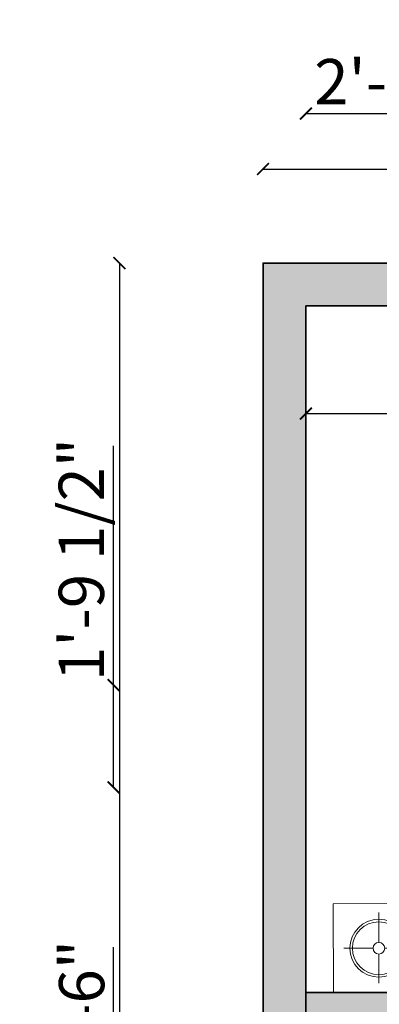
# Model space of a CAD drawing. Units: inches. Extents: x 1704 to 2334, y 1856 to 2559.
# Tile 4 of 10: x 1704 to 1779, y 2353 to 2559. Entities that reach past the tile are written whole.
import ezdxf

# ---------------------------------------------------------------- set-up
doc = ezdxf.new("R2010")
doc.units = ezdxf.units.IN
for name, color, linetype, lineweight in [('A-ANNO-DIMS', 2, 'Continuous', 18), ('A-WALL', 7, 'Continuous', 35), ('BEDS', 17, 'Continuous', 18)]:
    doc.layers.add(name, color=color, linetype=linetype, lineweight=lineweight)
doc.layers.add('A-WALL-PATT', color=18, linetype='Continuous', lineweight=13, true_color=0x000000)
doc.styles.get("Standard").update_dxf_attribs({"font": 'arial.ttf'})
doc.dimstyles.new('ISO-25', dxfattribs={"dimtxt": 9.5, "dimasz": 2.5, "dimexe": 1.25, "dimexo": 0.625, "dimtad": 1, "dimdec": 0, "dimlunit": 4, "dimtxsty": 'Standard', "dimblk": 'ARCHTICK', "dimcen": 2.5, "dimse1": 1, "dimse2": 1, "dimclrd": 3, "dimadec": 0, "dimazin": 0, "dimtfac": 1, "dimtdec": 0, "dimtmove": 0, "dimatfit": 3, "dimfxl": 1, "dimarcsym": 0})

# ---------------------------------------------------------------- blocks, each defined once
blk = doc.blocks.new('A$C77DF40FE')
for p, q in [((0.5, 2.6723), (0, 2.6723)), ((0, 2.6723), (0, 2.1723)), ((0.226, 2.4949), (0.226, 2.6594)), ((0.5, 2.1723), (0.5, 2.6723)), ((0.5839, 2.6714), (2.0097, 2.6714)), ((2.0936, 2.1723), (2.0936, 2.6723)), ((2.0936, 2.6723), (2.5936, 2.6723)), ((2.5936, 2.6723), (2.5936, 2.1723)), ((0.5339, 0.6344), (0.5339, 2.6214)), ((0.5839, 2.6214), (2.0097, 2.6214)), ((0.5839, 0.6344), (0.5839, 2.6214)), ((2.0097, 2.6214), (2.0097, 0.6344)), ((2.0597, 2.6214), (2.0597, 0.6344)), ((2.3379, 2.4554), (2.3379, 2.6199)), ((0.6508, 2.5603), (0.6508, 2.2403)), ((1.2408, 2.5803), (0.6708, 2.5803)), ((1.2608, 2.2403), (1.2608, 2.5603)), ((1.3355, 2.5603), (1.3355, 2.2403)), ((1.9255, 2.5803), (1.3555, 2.5803)), ((1.9455, 2.2403), (1.9455, 2.5603)), ((0.0287, 2.4621), (0.1932, 2.4621)), ((0.2588, 2.4621), (0.4233, 2.4621)), ((0.226, 2.261), (0.226, 2.4293)), ((0.4809, 2.3823), (0.4746, 2.3757)), ((0.4873, 2.387), (0.4809, 2.3823)), ((0.4937, 2.3899), (0.4873, 2.387)), ((0.5, 2.3914), (0.4937, 2.3899)), ((0.506, 2.3917), (0.5, 2.3914)), ((0.5117, 2.391), (0.506, 2.3917)), ((0.5168, 2.3897), (0.5117, 2.391)), ((0.5212, 2.3878), (0.5168, 2.3897)), ((0.5205, 2.3816), (0.5202, 2.3804)), ((0.5202, 2.3804), (0.5202, 2.379)), ((0.5202, 2.379), (0.5206, 2.3777)), ((0.521, 2.3828), (0.5205, 2.3816)), ((0.5219, 2.3839), (0.521, 2.3828)), ((0.5248, 2.3858), (0.5212, 2.3878)), ((0.523, 2.3849), (0.5219, 2.3839)), ((0.5244, 2.3856), (0.523, 2.3849)), ((0.5261, 2.3861), (0.5244, 2.3856)), ((0.5277, 2.3836), (0.5248, 2.3858)), ((0.5279, 2.3864), (0.5261, 2.3861)), ((0.5298, 2.3813), (0.5277, 2.3836)), ((0.5298, 2.3864), (0.5279, 2.3864)), ((0.5318, 2.3861), (0.5298, 2.3864)), ((0.5313, 2.3792), (0.5298, 2.3813)), ((0.5322, 2.3771), (0.5313, 2.3792)), ((0.5338, 2.3855), (0.5318, 2.3861)), ((0.5356, 2.3846), (0.5338, 2.3855)), ((0.5373, 2.3832), (0.5356, 2.3846)), ((0.5387, 2.3815), (0.5373, 2.3832)), ((0.5399, 2.3794), (0.5387, 2.3815)), ((0.5407, 2.377), (0.5399, 2.3794)), ((2.3051, 2.4226), (2.1406, 2.4226)), ((2.3379, 2.2215), (2.3379, 2.3898)), ((2.5352, 2.4226), (2.3707, 2.4226)), ((0.2338, 2.3688, 10.4), (0.2338, 2.1957, 10.4)), ((0.4828, 2.3788, 10.4), (0.2438, 2.3788, 10.4)), ((0.2538, 2.353, 10.4), (0.2538, 2.3215, 10.4)), ((0.4656, 2.363, 10.4), (0.2638, 2.363, 10.4)), ((0.4756, 2.3215, 10.4), (0.4756, 2.353, 10.4)), ((0.4767, 2.3409), (0.4876, 2.34)), ((0.4876, 2.34), (0.4961, 2.3402)), ((0.4928, 2.1957, 10.4), (0.4928, 2.3688, 10.4)), ((0.4961, 2.3402), (0.5023, 2.3413)), ((0.502, 2.3463), (0.5017, 2.3431)), ((0.5017, 2.3431), (0.5018, 2.3398)), ((0.5018, 2.3398), (0.5023, 2.3365)), ((0.5026, 2.3491), (0.502, 2.3463)), ((0.5023, 2.3413), (0.5067, 2.3431)), ((0.5023, 2.3365), (0.5031, 2.3334)), ((0.5035, 2.3514), (0.5026, 2.3491)), ((0.5031, 2.3334), (0.5043, 2.3309)), ((0.5047, 2.3531), (0.5035, 2.3514)), ((0.5043, 2.3309), (0.506, 2.329)), ((0.5059, 2.3542), (0.5047, 2.3531)), ((0.5073, 2.3548), (0.5059, 2.3542)), ((0.506, 2.329), (0.5081, 2.328)), ((0.5067, 2.3431), (0.5095, 2.3452)), ((0.5086, 2.3549), (0.5073, 2.3548)), ((0.5081, 2.328), (0.5106, 2.328)), ((0.5097, 2.3544), (0.5086, 2.3549)), ((0.5095, 2.3452), (0.511, 2.3475)), ((0.5107, 2.3534), (0.5097, 2.3544)), ((0.5106, 2.328), (0.5134, 2.3288)), ((0.5113, 2.3518), (0.5107, 2.3534)), ((0.511, 2.3475), (0.5115, 2.3498)), ((0.5115, 2.3498), (0.5113, 2.3518)), ((0.5134, 2.3288), (0.5163, 2.3304)), ((0.5163, 2.3304), (0.5193, 2.3325)), ((0.5193, 2.3325), (0.5222, 2.3349)), ((0.5206, 2.3777), (0.5213, 2.3764)), ((0.5213, 2.3764), (0.5224, 2.3752)), ((0.5222, 2.3349), (0.5249, 2.3374)), ((0.5224, 2.3752), (0.5237, 2.374)), ((0.5237, 2.374), (0.5252, 2.3731)), ((0.5249, 2.3374), (0.5271, 2.3398)), ((0.5252, 2.3731), (0.5268, 2.3723)), ((0.5268, 2.3723), (0.5283, 2.3719)), ((0.5271, 2.3398), (0.5288, 2.3419)), ((0.5283, 2.3719), (0.5297, 2.3717)), ((0.5288, 2.3419), (0.5299, 2.3436)), ((0.5297, 2.3717), (0.531, 2.372)), ((0.5299, 2.3436), (0.5305, 2.3449)), ((0.53, 2.3482), (0.5302, 2.3488)), ((0.5301, 2.3477), (0.53, 2.3482)), ((0.5303, 2.3472), (0.5301, 2.3477)), ((0.5302, 2.3488), (0.5308, 2.3495)), ((0.5306, 2.3466), (0.5303, 2.3472)), ((0.5305, 2.3449), (0.5307, 2.3459)), ((0.5307, 2.3459), (0.5306, 2.3466)), ((0.5308, 2.3495), (0.5317, 2.3504)), ((0.531, 2.372), (0.5319, 2.3726)), ((0.5317, 2.3504), (0.5329, 2.3515)), ((0.5319, 2.3726), (0.5325, 2.3738)), ((0.5326, 2.3753), (0.5322, 2.3771)), ((0.5325, 2.3738), (0.5326, 2.3753)), ((0.5329, 2.3515), (0.5342, 2.3528)), ((0.5342, 2.3528), (0.5356, 2.3543)), ((0.5356, 2.3543), (0.537, 2.3561)), ((0.537, 2.3561), (0.5383, 2.3581)), ((0.5383, 2.3581), (0.5394, 2.3604)), ((0.5394, 2.3604), (0.5403, 2.3629)), ((0.5403, 2.3629), (0.5409, 2.3657)), ((0.5412, 2.3743), (0.5407, 2.377)), ((0.5409, 2.3657), (0.5413, 2.3686)), ((0.5414, 2.3715), (0.5412, 2.3743)), ((0.5413, 2.3686), (0.5414, 2.3715)), ((0.2638, 2.3115, 10.4), (0.4656, 2.3115, 10.4)), ((0.6708, 2.2203), (1.2408, 2.2203)), ((1.3555, 2.2203), (1.9255, 2.2203)), ((0, 2.1723), (0.5, 2.1723)), ((0.2438, 2.1857, 10.4), (0.4828, 2.1857, 10.4)), ((2.5936, 2.1723), (2.0936, 2.1723)), ((1.5773, 2.1205), (1.0147, 2.1205)), ((0.1072, 1.9057), (0.0269, 1.9485)), ((0.0644, 1.9807), (0.1019, 1.9003)), ((0.1072, 1.986), (0.1072, 1.911)), ((0.134, 1.9753), (0.134, 1.9057)), ((0.1554, 1.9914), (0.1554, 1.911)), ((0.1792, 1.9138), (0.1849, 1.9847)), ((0.2134, 1.9138), (0.219, 1.9847)), ((0.251, 1.9118), (0.2494, 1.9865)), ((0.2748, 1.9118), (0.2691, 1.9849)), ((0.2899, 1.9138), (0.2956, 1.9847)), ((0.3277, 1.9118), (0.3219, 1.9849)), ((0.3539, 1.9118), (0.3522, 1.9865)), ((0.3766, 1.9138), (0.3822, 1.9847)), ((0.4142, 1.9118), (0.4126, 1.9865)), ((0.438, 1.9118), (0.4323, 1.9849)), ((0.4531, 1.9138), (0.4588, 1.9847)), ((0.4873, 1.9138), (0.493, 1.9847)), ((0.5249, 1.9118), (0.5233, 1.9865)), ((0.0195, 1.8887), (0.0942, 1.8903)), ((0.1019, 1.9003), (0.0269, 1.9003)), ((0.1002, 1.8885), (0.1002, 0.0935)), ((0.3112, 1.9057), (0.1019, 1.9057)), ((0.1019, 1.9057), (0.1019, 1.8628)), ((0.5301, 1.9057), (0.3112, 1.9057)), ((0.6051, 1.925), (0.7457, 1.7234)), ((1.9869, 1.925), (1.8463, 1.7234)), ((0.0227, 1.8712), (0.0957, 1.8769)), ((0.0247, 1.8561), (0.0955, 1.8504)), ((0.0227, 1.7843), (0.0974, 1.786)), ((0.0247, 1.8219), (0.0955, 1.8163)), ((0.3112, 1.8116), (0.1852, 1.8116)), ((0.1852, 1.8116), (0.1852, 0.187)), ((0.3112, 1.7816), (0.2152, 1.7816)), ((0.2152, 1.7816), (0.2152, 0.217)), ((0.5339, 1.8116), (0.3112, 1.8116)), ((0.5339, 1.7816), (0.3112, 1.7816)), ((0.3909, 1.7821), (0.5339, 1.398)), ((0.0227, 1.7605), (0.0957, 1.7662)), ((0.0247, 1.7454), (0.0955, 1.7397)), ((0.0247, 1.708), (0.0955, 1.7023)), ((0.0247, 1.6819), (0.0955, 1.6762)), ((0.0227, 1.6443), (0.0974, 1.6459)), ((0.0227, 1.6205), (0.0957, 1.6262)), ((0.0247, 1.6054), (0.0955, 1.5997)), ((0.0227, 1.5505), (0.0974, 1.5521)), ((0.0247, 1.5881), (0.0955, 1.5824)), ((0.0227, 1.5266), (0.0957, 1.5324)), ((0.0247, 1.5116), (0.0955, 1.5059)), ((0.0227, 1.4397), (0.0974, 1.4414)), ((0.0247, 1.4774), (0.0955, 1.4717)), ((0.0227, 1.4159), (0.0957, 1.4217)), ((0.0247, 1.4008), (0.0955, 1.3952)), ((0.0247, 1.3634), (0.0955, 1.3577)), ((0.0247, 1.3374), (0.0955, 1.3317)), ((0.0227, 1.2997), (0.0974, 1.3014)), ((0.0227, 1.2759), (0.0957, 1.2816)), ((0.0247, 1.2608), (0.0955, 1.2551)), ((0.0247, 1.2266), (0.0955, 1.221)), ((0.0227, 1.189), (0.0974, 1.1906)), ((0.0227, 1.1652), (0.0957, 1.1709)), ((0.0227, 1.1414), (0.0957, 1.1471)), ((0.0247, 1.1163), (0.0955, 1.1106)), ((0.5339, 1.1132), (0.2152, 1.1479)), ((0.0227, 1.0786), (0.0974, 1.0803)), ((0.0227, 1.0548), (0.0957, 1.0606)), ((0.0247, 1.0397), (0.0955, 1.0341)), ((0.0247, 1.0055), (0.0955, 0.9999)), ((0.5339, 0.7837), (0.2152, 1.0221)), ((0.0227, 0.9679), (0.0974, 0.9696)), ((0.0227, 0.9441), (0.0957, 0.9498)), ((0.0247, 0.929), (0.0955, 0.9233)), ((0.0247, 0.8916), (0.0955, 0.8859)), ((0.0247, 0.8655), (0.0955, 0.8599)), ((0.0227, 0.8279), (0.0974, 0.8295)), ((0.0227, 0.8041), (0.0957, 0.8098)), ((0.0247, 0.789), (0.0955, 0.7833)), ((0.0247, 0.7548), (0.0955, 0.7491)), ((0.0227, 0.7172), (0.0974, 0.7188)), ((0.0227, 0.6933), (0.0957, 0.6991)), ((0.0247, 0.6783), (0.0955, 0.6726)), ((0.0247, 0.6408), (0.0955, 0.6352)), ((2.0097, 0.6344), (0.5839, 0.6344)), ((0.0227, 0.6032), (0.0974, 0.6048)), ((0.0227, 0.5794), (0.0957, 0.5851)), ((0.0247, 0.5643), (0.0955, 0.5586)), ((2.0097, 0.5844), (0.5839, 0.5844)), ((1.2963, 0.2134), (0.8003, 0.5844)), ((0.8369, 0.5844), (0.975, 0.2134)), ((1.6139, 0.217), (1.6139, 0.5844)), ((1.6439, 0.187), (1.6439, 0.5844)), ((1.7439, 0.087), (1.7439, 0.5844)), ((1.8197, 0.5605), (1.7489, 0.5548)), ((0.0247, 0.5301), (0.0955, 0.5244)), ((1.8218, 0.5229), (1.7471, 0.5245)), ((1.8218, 0.499), (1.7487, 0.5048)), ((0.0227, 0.4925), (0.0974, 0.4941)), ((0.0227, 0.4687), (0.0957, 0.4744)), ((0.0247, 0.4536), (0.0955, 0.4479)), ((1.8197, 0.4839), (1.7489, 0.4783)), ((1.8197, 0.453), (1.7489, 0.4474)), ((0.0247, 0.4227), (0.0955, 0.417)), ((1.8197, 0.4168), (1.7489, 0.4111)), ((0.0227, 0.3367), (0.0957, 0.3424)), ((0.0247, 0.3864), (0.0955, 0.3807)), ((1.8218, 0.3671), (1.7487, 0.3728)), ((1.8197, 0.352), (1.7489, 0.3463)), ((0.0247, 0.3216), (0.0955, 0.3159)), ((0.0247, 0.2842), (0.0955, 0.2785)), ((1.8197, 0.3146), (1.7489, 0.3089)), ((1.7492, 0.2844), (1.8223, 0.2787)), ((0.0227, 0.2465), (0.0974, 0.2482)), ((0.0227, 0.2227), (0.0957, 0.2285)), ((1.7492, 0.2606), (1.824, 0.2589)), ((1.7513, 0.223), (1.8221, 0.2286)), ((0.1019, 0.1857), (0.0216, 0.1857)), ((0.0247, 0.2076), (0.0955, 0.202)), ((0.1852, 0.187), (0.3112, 0.187)), ((0.2152, 0.217), (0.3112, 0.217)), ((0.3112, 0.217), (1.6139, 0.217)), ((0.3112, 0.187), (1.6439, 0.187)), ((1.7492, 0.1737), (1.8223, 0.1679)), ((1.7513, 0.1888), (1.8221, 0.1944)), ((0.1019, 0.1535), (0.0269, 0.1482)), ((0.1019, 0.116), (0.0269, 0.1214)), ((1.7492, 0.1499), (1.824, 0.1482)), ((1.7513, 0.1122), (1.8221, 0.1179)), ((0.0965, 0.0946), (0.0269, 0.0303)), ((0.1019, 0.0892), (0.0269, 0.0892)), ((0.1019, 0.0946), (0.0751, 0.0089)), ((0.1002, 0.0935), (0.3112, 0.0935)), ((0.107, 0.0096), (0.1126, 0.0804)), ((0.1446, 0.0075), (0.1429, 0.0823)), ((0.1684, 0.0075), (0.1627, 0.0806)), ((0.1835, 0.0096), (0.1892, 0.0804)), ((0.2209, 0.0096), (0.2266, 0.0804)), ((0.247, 0.0096), (0.2527, 0.0804)), ((0.2846, 0.0075), (0.283, 0.0823)), ((0.3084, 0.0075), (0.3027, 0.0806)), ((0.3112, 0.0935), (1.0155, 0.0935)), ((0.3151, 0.0075), (0.3112, 0.0565)), ((0.3301, 0.0096), (0.3358, 0.0804)), ((0.3676, 0.0096), (0.3732, 0.0804)), ((0.3936, 0.0096), (0.3993, 0.0804)), ((0.4313, 0.0075), (0.4296, 0.0823)), ((0.4551, 0.0075), (0.4493, 0.0806)), ((0.4702, 0.0096), (0.4758, 0.0804)), ((0.5043, 0.0096), (0.51, 0.0804)), ((0.542, 0.0075), (0.5403, 0.0823)), ((0.5658, 0.0075), (0.56, 0.0806)), ((0.5896, 0.0075), (0.5838, 0.0806)), ((0.6147, 0.0096), (0.6204, 0.0804)), ((0.6523, 0.0075), (0.6507, 0.0823)), ((0.6762, 0.0075), (0.6704, 0.0806)), ((0.6912, 0.0096), (0.6969, 0.0804)), ((0.7254, 0.0096), (0.7311, 0.0804)), ((0.7631, 0.0075), (0.7614, 0.0823)), ((0.7869, 0.0075), (0.7811, 0.0806)), ((0.802, 0.0096), (0.8076, 0.0804)), ((0.8394, 0.0096), (0.8451, 0.0804)), ((0.8654, 0.0096), (0.8711, 0.0804)), ((0.9031, 0.0075), (0.9014, 0.0823)), ((0.9269, 0.0075), (0.9212, 0.0806)), ((0.942, 0.0096), (0.9477, 0.0804)), ((0.9762, 0.0096), (0.9818, 0.0804)), ((1.0138, 0.0075), (1.0122, 0.0823)), ((1.0155, 0.0935), (1.7355, 0.0935)), ((1.0376, 0.0075), (1.0319, 0.0806)), ((1.0527, 0.0096), (1.0584, 0.0804)), ((1.0901, 0.0096), (1.0958, 0.0804)), ((1.1278, 0.0075), (1.1261, 0.0823)), ((1.1516, 0.0075), (1.1459, 0.0806)), ((1.1667, 0.0096), (1.1724, 0.0804)), ((1.2009, 0.0096), (1.2065, 0.0804)), ((1.2385, 0.0075), (1.2368, 0.0823)), ((1.2623, 0.0075), (1.2566, 0.0806)), ((1.2774, 0.0096), (1.2831, 0.0804)), ((1.3083, 0.0096), (1.314, 0.0804)), ((1.3446, 0.0096), (1.3503, 0.0804)), ((1.3943, 0.0075), (1.3885, 0.0806)), ((1.4094, 0.0096), (1.415, 0.0804)), ((1.4468, 0.0096), (1.4525, 0.0804)), ((1.4844, 0.0075), (1.4828, 0.0823)), ((1.5083, 0.0075), (1.5025, 0.0806)), ((1.5233, 0.0096), (1.529, 0.0804)), ((1.5575, 0.0096), (1.5632, 0.0804)), ((1.5951, 0.0075), (1.5935, 0.0823)), ((1.619, 0.0075), (1.6132, 0.0806)), ((1.6341, 0.0096), (1.6397, 0.0804)), ((1.665, 0.0096), (1.6706, 0.0804)), ((1.6831, 0.0096), (1.6888, 0.0804)), ((1.7162, 0.0857), (1.7162, 0)), ((1.7323, 0.0911), (1.7269, 0.0107)), ((1.743, 0.0857), (1.8126, 0.0054)), ((1.7483, 0.0911), (1.8233, 0.0322)), ((1.7483, 0.0857), (1.7537, 0.0054)), ((1.7513, 0.0858), (1.8221, 0.0915))]:
    blk.add_line(p, q)
for centre, radius in [((0.226, 2.4621), 0.1629), ((0.226, 2.4621), 0.1484), ((2.3379, 2.4226), 0.1629), ((2.3379, 2.4226), 0.1484), ((0.226, 2.4621), 0.0328), ((2.3379, 2.4226), 0.0328), ((0.2896, 2.2801, 10.4), 0.00858), ((0.3196, 2.2801, 10.4), 0.00858), ((0.3554, 2.2801, 10.4), 0.00858), ((0.3855, 2.2801, 10.4), 0.00858), ((0.2896, 2.25, 10.4), 0.00858), ((0.2896, 2.2186, 10.4), 0.00858), ((0.3196, 2.25, 10.4), 0.00858), ((0.3196, 2.2186, 10.4), 0.00858), ((0.3554, 2.25, 10.4), 0.00858), ((0.3554, 2.2186, 10.4), 0.00858), ((0.3855, 2.25, 10.4), 0.00858), ((0.3855, 2.2186, 10.4), 0.00858)]:
    blk.add_circle(centre, radius)
for centre, radius, start, end in [((0.5839, 2.6214), 0.05, 90, 180), ((2.0097, 2.6214), 0.05, 0, 90), ((0.6708, 2.5603), 0.02, 90, 180), ((0.9635, 1.1066), 1.4427, 78.1527, 102.4906), ((0.9287, 0.5819), 1.9884, 80.4201, 97.9672), ((1.4247, 2.3742), 0.7696, 164.6112, 191.5679), ((1.0701, 2.3966), 0.3942, 152.5365, 206.92), ((1.6628, 2.4129), 0.928, 169.6087, 191.899), ((1.6628, 2.4129), 0.908, 169.6087, 191.899), ((2.7571, 2.4533), 1.9523, 176.3947, 186.8195), ((2.7571, 2.4533), 1.9323, 176.3947, 186.8195), ((3.9259, 2.3685), 3.0367, 176.1432, 182.775), ((3.9259, 2.3685), 3.0167, 176.1432, 182.775), ((-2.0216, 2.3685), 3.0167, 357.225, 3.8568), ((-2.0216, 2.3685), 3.0367, 357.225, 3.8568), ((-0.8455, 2.4533), 1.9323, 353.1805, 3.6053), ((-0.8455, 2.4533), 1.9523, 353.1805, 3.6053), ((0.2489, 2.4129), 0.908, 348.101, 10.3913), ((0.2489, 2.4129), 0.928, 348.101, 10.3913), ((0.8416, 2.3966), 0.3942, 333.08, 27.4635), ((0.4869, 2.3742), 0.7696, 348.4321, 15.3888), ((1.2408, 2.5603), 0.02, 0, 90), ((1.3555, 2.5603), 0.02, 90, 180), ((1.6482, 1.1066), 1.4427, 78.1527, 102.4906), ((1.6135, 0.5819), 1.9884, 80.4201, 97.9672), ((2.1094, 2.3742), 0.7696, 164.6112, 191.5679), ((1.7548, 2.3966), 0.3942, 152.5365, 206.92), ((2.3475, 2.4129), 0.928, 169.6087, 191.899), ((2.3475, 2.4129), 0.908, 169.6087, 191.899), ((3.4419, 2.4533), 1.9523, 176.3947, 186.8195), ((3.4419, 2.4533), 1.9323, 176.3947, 186.8195), ((4.6106, 2.3685), 3.0367, 176.1432, 182.775), ((4.6106, 2.3685), 3.0167, 176.1432, 182.775), ((-1.3369, 2.3685), 3.0167, 357.225, 3.8568), ((-1.3369, 2.3685), 3.0367, 357.225, 3.8568), ((-0.1608, 2.4533), 1.9323, 353.1805, 3.6053), ((-0.1608, 2.4533), 1.9523, 353.1805, 3.6053), ((0.9336, 2.4129), 0.908, 348.101, 10.3913), ((0.9336, 2.4129), 0.928, 348.101, 10.3913), ((1.5263, 2.3966), 0.3942, 333.08, 27.4635), ((1.1716, 2.3742), 0.7696, 348.4321, 15.3888), ((1.9255, 2.5603), 0.02, 0, 90), ((0.9445, -2.3575), 4.8647, 86.2671, 93.4563), ((1.6292, -2.3575), 4.8647, 86.2671, 93.4563), ((0.9561, -3.928), 6.3765, 87.24779, 92.75221), ((0.9445, -2.3575), 4.8447, 86.2671, 93.4563), ((1.6408, -3.928), 6.3765, 87.24779, 92.75221), ((1.6292, -2.3575), 4.8447, 86.2671, 93.4563), ((0.9561, -3.928), 6.3565, 87.24779, 92.75221), ((0.9561, 8.7285), 6.3565, 267.24779, 272.75221), ((1.6408, -3.928), 6.3565, 87.24779, 92.75221), ((1.6408, 8.7285), 6.3565, 267.24779, 272.75221), ((0.2438, 2.3688, 10.4), 0.01, 90, 180), ((0.2638, 2.353, 10.4), 0.01, 90, 180), ((0.4656, 2.353, 10.4), 0.01, 0, 90), ((0.4828, 2.3688, 10.4), 0.01, 0, 90), ((0.9561, 8.7285), 6.3765, 267.24779, 272.75221), ((0.9445, 7.158), 4.8447, 266.5437, 273.7329), ((1.6408, 8.7285), 6.3765, 267.24779, 272.75221), ((1.6292, 7.158), 4.8447, 266.5437, 273.7329), ((0.2638, 2.3215, 10.4), 0.01, 180, 270), ((0.43, 2.2801, 10.4), 0.00304, 140.3607, 180), ((0.43, 2.2801, 10.4), 0.00304, 180, 219.6393), ((0.434, 2.2768, 10.4), 0.00822, 116.5651, 140.3607), ((0.434, 2.2834, 10.4), 0.00822, 219.6393, 243.4349), ((0.4367, 2.2714, 10.4), 0.0142, 101.7009, 116.5651), ((0.4367, 2.2887, 10.4), 0.0142, 243.4349, 258.2991), ((0.4384, 2.263, 10.4), 0.0228, 90, 101.7009), ((0.4384, 2.2972, 10.4), 0.0228, 258.2991, 270), ((0.4384, 2.263, 10.4), 0.0228, 78.2991, 90), ((0.4384, 2.2972, 10.4), 0.0228, 270, 281.7009), ((0.4402, 2.2714, 10.4), 0.0142, 63.4349, 78.2991), ((0.4402, 2.2887, 10.4), 0.0142, 281.7009, 296.5651), ((0.4428, 2.2768, 10.4), 0.00822, 39.6393, 63.4349), ((0.4428, 2.2834, 10.4), 0.00822, 296.5651, 320.3607), ((0.4468, 2.2801, 10.4), 0.00304, 0, 39.6393), ((0.4468, 2.2801, 10.4), 0.00304, 320.3607, 0), ((0.4656, 2.3215, 10.4), 0.01, 270, 0), ((0.9445, 7.158), 4.8647, 266.5437, 273.7329), ((0.9635, 3.6939), 1.4427, 257.5094, 281.8473), ((1.6292, 7.158), 4.8647, 266.5437, 273.7329), ((1.6482, 3.6939), 1.4427, 257.5094, 281.8473), ((0.43, 2.2586, 10.4), 0.00304, 140.3607, 180), ((0.43, 2.2586, 10.4), 0.00304, 180, 219.6393), ((0.43, 2.2386, 10.4), 0.00304, 140.3607, 180), ((0.43, 2.2386, 10.4), 0.00304, 180, 219.6393), ((0.434, 2.2553, 10.4), 0.00822, 116.5651, 140.3607), ((0.434, 2.2619, 10.4), 0.00822, 219.6393, 243.4349), ((0.434, 2.2353, 10.4), 0.00822, 116.5651, 140.3607), ((0.434, 2.2419, 10.4), 0.00822, 219.6393, 243.4349), ((0.4314, 2.2186, 10.4), 0.00304, 140.3607, 180), ((0.4314, 2.2186, 10.4), 0.00304, 180, 219.6393), ((0.4354, 2.2153, 10.4), 0.00822, 116.5651, 140.3607), ((0.4354, 2.2219, 10.4), 0.00822, 219.6393, 243.4349), ((0.4367, 2.25, 10.4), 0.0142, 101.7009, 116.5651), ((0.4367, 2.2673, 10.4), 0.0142, 243.4349, 258.2991), ((0.4367, 2.23, 10.4), 0.0142, 101.7009, 116.5651), ((0.4367, 2.2472, 10.4), 0.0142, 243.4349, 258.2991), ((0.4381, 2.2099, 10.4), 0.0142, 101.7009, 116.5651), ((0.4381, 2.2272, 10.4), 0.0142, 243.4349, 258.2991), ((0.4384, 2.2415, 10.4), 0.0228, 90, 101.7009), ((0.4384, 2.2757, 10.4), 0.0228, 258.2991, 270), ((0.4384, 2.2215, 10.4), 0.0228, 90, 101.7009), ((0.4384, 2.2557, 10.4), 0.0228, 258.2991, 270), ((0.4398, 2.2015, 10.4), 0.0228, 90, 101.7009), ((0.4398, 2.2357, 10.4), 0.0228, 258.2991, 270), ((0.4384, 2.2415, 10.4), 0.0228, 78.2991, 90), ((0.4384, 2.2757, 10.4), 0.0228, 270, 281.7009), ((0.4384, 2.2215, 10.4), 0.0228, 78.2991, 90), ((0.4384, 2.2557, 10.4), 0.0228, 270, 281.7009), ((0.4398, 2.2015, 10.4), 0.0228, 78.2991, 90), ((0.4398, 2.2357, 10.4), 0.0228, 270, 281.7009), ((0.4402, 2.25, 10.4), 0.0142, 63.4349, 78.2991), ((0.4402, 2.2673, 10.4), 0.0142, 281.7009, 296.5651), ((0.4402, 2.23, 10.4), 0.0142, 63.4349, 78.2991), ((0.4402, 2.2472, 10.4), 0.0142, 281.7009, 296.5651), ((0.4416, 2.2099, 10.4), 0.0142, 63.4349, 78.2991), ((0.4416, 2.2272, 10.4), 0.0142, 281.7009, 296.5651), ((0.4428, 2.2553, 10.4), 0.00822, 39.6393, 63.4349), ((0.4428, 2.2619, 10.4), 0.00822, 296.5651, 320.3607), ((0.4428, 2.2353, 10.4), 0.00822, 39.6393, 63.4349), ((0.4428, 2.2419, 10.4), 0.00822, 296.5651, 320.3607), ((0.4443, 2.2153, 10.4), 0.00822, 39.6393, 63.4349), ((0.4443, 2.2219, 10.4), 0.00822, 296.5651, 320.3607), ((0.4468, 2.2586, 10.4), 0.00304, 0, 39.6393), ((0.4468, 2.2586, 10.4), 0.00304, 320.3607, 0), ((0.4468, 2.2386, 10.4), 0.00304, 0, 39.6393), ((0.4468, 2.2386, 10.4), 0.00304, 320.3607, 0), ((0.4483, 2.2186, 10.4), 0.00304, 0, 39.6393), ((0.4483, 2.2186, 10.4), 0.00304, 320.3607, 0), ((0.6708, 2.2403), 0.02, 180, 270), ((0.9287, 4.2186), 1.9884, 262.0328, 279.5799), ((1.2408, 2.2403), 0.02, 270, 0), ((1.3555, 2.2403), 0.02, 180, 270), ((1.6135, 4.2186), 1.9884, 262.0328, 279.5799), ((1.9255, 2.2403), 0.02, 270, 0), ((0.2438, 2.1957, 10.4), 0.01, 180, 270), ((0.4828, 2.1957, 10.4), 0.01, 270, 0), ((1.1396, 1.3485), 0.782, 99.1908, 132.5116), ((1.3217, 1.6229), 0.5847, 121.6676, 170.1065), ((10.1174, 1.2237), 9.161, 174.43278, 183.67204), ((1.3248, -2.1722), 4.2793, 86.1532, 94.7091), ((10.2564, 1.2237), 9.181, 174.43278, 183.67204), ((10.2564, 1.2237), 9.161, 174.43278, 183.67204), ((16.3019, 1.253), 15.0916, 176.72768, 182.32074), ((16.3019, 1.253), 15.0716, 176.72768, 182.32074), ((-13.7099, 1.253), 15.0716, 357.67926, 3.27232), ((-13.7099, 1.253), 15.0916, 357.67926, 3.27232), ((-7.6644, 1.2237), 9.161, 356.32796, 5.56722), ((-7.6644, 1.2237), 9.181, 356.32796, 5.56722), ((1.2703, 1.6229), 0.5847, 9.8935, 58.3324), ((1.4523, 1.3485), 0.782, 47.4884, 80.8092), ((-7.5254, 1.2237), 9.161, 356.32796, 5.55658), ((10.1174, 1.2237), 9.181, 174.54912, 183.67204), ((1.3248, -2.1722), 4.2593, 85.7473, 95.1159), ((-7.5254, 1.2237), 9.181, 356.32796, 5.45088), ((4.947, 1.2796), 4.1406, 170.0939, 188.8179), ((1.3657, -2.1044), 4.1088, 84.9619, 97.1707), ((-2.355, 1.2796), 4.1406, 351.1821, 9.9061), ((4.947, 1.2796), 4.1606, 170.6272, 188.8179), ((1.3657, -2.1044), 4.0888, 84.7053, 97.4283), ((-2.355, 1.2796), 4.1606, 351.1821, 9.3728), ((7.8077, 1.3061), 7.2149, 175.27403, 185.28261), ((7.8077, 1.3061), 7.1949, 175.41729, 185.28261), ((1.3142, -3.5764), 5.4671, 84.8953, 95.5052), ((-5.2157, 1.3061), 7.1949, 354.71739, 4.58271), ((-5.2157, 1.3061), 7.2149, 354.71739, 4.72597), ((1.3142, -3.5764), 5.4671, 96.9078, 97.6924), ((1.3142, -3.5764), 5.4471, 96.796, 97.6924), ((1.3142, -3.5764), 5.4471, 84.7792, 95.6214), ((1.3142, -3.5764), 5.4471, 82.7025, 83.5609), ((1.3142, -3.5764), 5.4671, 82.7025, 83.4474), ((1.2659, -7.4764), 9.2344, 85.41732, 94.18368), ((1.2659, -7.4764), 9.2144, 85.41732, 94.18368), ((4.8527, 1.2796), 4.1606, 173.3677, 188.8179), ((4.8527, 1.2796), 4.1406, 173.6812, 188.8179), ((-2.2608, 1.2796), 4.1406, 351.1821, 6.3188), ((-2.2608, 1.2796), 4.1606, 351.1821, 6.6323), ((1.4138, -15.5462), 17.172, 88.01473, 92.775), ((1.4138, -15.5462), 17.152, 88.01473, 92.775), ((1.4138, -15.6721), 17.172, 88.01473, 92.775), ((1.4138, -15.6721), 17.152, 88.01473, 92.775), ((1.4138, 18.4566), 17.172, 267.225, 271.98527), ((1.4138, 18.4566), 17.152, 267.225, 271.98527), ((1.4138, 18.3004), 17.152, 267.225, 271.98527), ((1.4138, 18.3004), 17.172, 267.225, 271.98527), ((1.2659, 10.2305), 9.2344, 265.81632, 274.58268), ((1.2659, 10.2305), 9.2144, 265.81632, 274.58268), ((1.3142, 6.3306), 5.4471, 262.3076, 277.2975), ((1.3657, 4.8586), 4.0888, 259.0794, 278.9327), ((1.3657, 4.8586), 4.1088, 259.0794, 278.9327), ((1.3248, 4.9264), 4.2593, 260.0761, 279.1287), ((1.3248, 4.9264), 4.2793, 260.0761, 279.1287), ((0.5839, 0.6344), 0.05, 180, 270), ((2.0097, 0.6344), 0.05, 270, 0)]:
    blk.add_arc(centre, radius, start, end)
for p in [(0.2895, 1.7311), (0.5004, 1.7457), (0.2895, 1.6873), (0.3179, 1.6946), (0.4274, 1.6581), (0.3471, 1.5195), (0.9622, 1.5058), (0.2822, 1.4684), (0.3471, 1.4684), (0.5004, 1.4684), (0.3471, 1.41), (0.4326, 1.3443), (0.4858, 1.3444), (0.4253, 1.3151), (0.5077, 1.286), (0.4253, 1.2495), (0.3041, 1.2057), (0.3909, 1.213), (0.4253, 1.1692), (0.3106, 1.0671), (0.4931, 1.0452), (0.4765, 0.9722), (0.3114, 0.7971), (0.4034, 0.7971), (0.4034, 0.7169), (0.4931, 0.7096), (0.4034, 0.6512), (0.4055, 0.6512), (0.4931, 0.5564), (0.4984, 0.5782), (1.3453, 0.5782), (1.1794, 0.5491), (1.1867, 0.5345), (1.4058, 0.5345), (1.7124, 0.5272), (0.5734, 0.4761), (0.6757, 0.4542), (1.0407, 0.4469), (1.2671, 0.4615), (0.3909, 0.4396), (0.5296, 0.4104), (0.7341, 0.4032), (1.1794, 0.4032), (1.5299, 0.4104), (1.6759, 0.4032), (0.2895, 0.3448), (0.7779, 0.3594), (1.2963, 0.3448), (1.4204, 0.3448), (1.4788, 0.3813), (0.3114, 0.3302), (0.5296, 0.2937), (0.6538, 0.2937), (0.8655, 0.2937), (1.0261, 0.3229), (1.5445, 0.2864), (1.7652, 0.2958), (1.2693, 0.1315), (0.6049, 0.0659), (0.8093, 0.0659), (1.3861, 0.0732), (1.5686, 0.0878), (0.4588, 0.0513)]:
    blk.add_point(p)
blk = doc.blocks.new('_ArchTick')
at = {"color": 0, "linetype": 'ByBlock', "const_width": 0.15}
blk.add_lwpolyline([(-0.5, -0.5), (0.5, 0.5)], dxfattribs=at)
blk = doc.blocks.new('*D12')
at = {"layer": 'A-ANNO-DIMS', "color": 0, "lineweight": -2, "transparency": 16777216}
blk.add_line((1764.01, 2476.46), (1922.01, 2476.46), dxfattribs=at)
at = {"layer": 'Defpoints', "color": 0, "transparency": 16777216}
for p in [(1922.01, 2476.46), (1764.01, 2468.82), (1922.01, 2468.82)]:
    blk.add_point(p, dxfattribs=at)
at = {"layer": 'A-ANNO-DIMS', "color": 0, "lineweight": -2, "transparency": 16777216, "xscale": 2.5, "yscale": 2.5, "zscale": 2.5, "rotation": 180}
blk.add_blockref('_ArchTick', (1764.01, 2476.46), dxfattribs=at)
at = {"layer": 'A-ANNO-DIMS', "color": 0, "lineweight": -2, "transparency": 16777216, "xscale": 2.5, "yscale": 2.5, "zscale": 2.5}
blk.add_blockref('_ArchTick', (1922.01, 2476.46), dxfattribs=at)
at = {"layer": 'A-ANNO-DIMS', "color": 0, "transparency": 16777216, "insert": (1843.01, 2481.94), "char_height": 9.5, "attachment_point": 5}
blk.add_mtext('13\'-2"', dxfattribs=at)
blk = doc.blocks.new('*D22')
at = {"layer": 'A-ANNO-DIMS', "color": 0, "lineweight": -2, "transparency": 16777216}
blk.add_line((1755.01, 2527.77), (2175.01, 2527.77), dxfattribs=at)
at = {"layer": 'Defpoints', "color": 0, "transparency": 16777216}
for p in [(2175.01, 2527.77), (1755.01, 2508.04), (2175.01, 2508.04)]:
    blk.add_point(p, dxfattribs=at)
at = {"layer": 'A-ANNO-DIMS', "color": 0, "lineweight": -2, "transparency": 16777216, "xscale": 2.5, "yscale": 2.5, "zscale": 2.5, "rotation": 180}
blk.add_blockref('_ArchTick', (1755.01, 2527.77), dxfattribs=at)
at = {"layer": 'A-ANNO-DIMS', "color": 0, "lineweight": -2, "transparency": 16777216, "xscale": 2.5, "yscale": 2.5, "zscale": 2.5}
blk.add_blockref('_ArchTick', (2175.01, 2527.77), dxfattribs=at)
at = {"layer": 'A-ANNO-DIMS', "color": 0, "transparency": 16777216, "insert": (1965.01, 2533.25), "char_height": 9.5, "attachment_point": 5}
blk.add_mtext("35'", dxfattribs=at)
blk = doc.blocks.new('*D23')
at = {"layer": 'A-ANNO-DIMS', "color": 0, "lineweight": -2, "transparency": 16777216}
blk.add_line((1724.87, 2508.04), (1724.87, 1968.04), dxfattribs=at)
at = {"layer": 'Defpoints', "color": 0, "transparency": 16777216}
for p in [(1755.01, 2508.04), (1724.87, 1968.04), (1755.01, 1968.04)]:
    blk.add_point(p, dxfattribs=at)
at = {"layer": 'A-ANNO-DIMS', "color": 0, "lineweight": -2, "transparency": 16777216, "xscale": 2.5, "yscale": 2.5, "zscale": 2.5}
for p, rotation in [((1724.87, 2508.04), 90), ((1724.87, 1968.04), 270)]:
    blk.add_blockref('_ArchTick', p, dxfattribs=dict(at, rotation=rotation))
at = {"layer": 'A-ANNO-DIMS', "color": 0, "transparency": 16777216, "insert": (1719.41, 2238.04), "char_height": 9.5, "attachment_point": 5, "rotation": 90}
blk.add_mtext("45'", dxfattribs=at)
blk = doc.blocks.new('*D43')
at = {"layer": 'A-ANNO-DIMS', "color": 3, "lineweight": -2, "transparency": 16777216}
blk.add_line((1764.01, 2539.39), (1796.13, 2539.39), dxfattribs=at)
at = {"layer": 'Defpoints', "color": 0, "transparency": 16777216}
for p in [(1796.13, 2539.39), (1764.01, 2148.04), (1796.13, 2148.04)]:
    blk.add_point(p, dxfattribs=at)
at = {"layer": 'A-ANNO-DIMS', "color": 3, "lineweight": -2, "transparency": 16777216, "xscale": 2.5, "yscale": 2.5, "zscale": 2.5, "rotation": 180}
blk.add_blockref('_ArchTick', (1764.01, 2539.39), dxfattribs=at)
at = {"layer": 'A-ANNO-DIMS', "color": 3, "lineweight": -2, "transparency": 16777216, "xscale": 2.5, "yscale": 2.5, "zscale": 2.5}
blk.add_blockref('_ArchTick', (1796.13, 2539.39), dxfattribs=at)
at = {"layer": 'A-ANNO-DIMS', "color": 0, "transparency": 16777216, "insert": (1780.07, 2544.86), "char_height": 9.5, "attachment_point": 5}
blk.add_mtext('2\'-8"', dxfattribs=at)
blk = doc.blocks.new('*D48')
at = {"layer": 'A-ANNO-DIMS', "color": 3, "lineweight": -2, "transparency": 16777216}
for p, q in [((1764.01, 2539.39), (1799.73, 2539.39)), ((1799.73, 2539.39), (1858.41, 2539.39))]:
    blk.add_line(p, q, dxfattribs=at)
at = {"layer": 'Defpoints', "color": 0, "transparency": 16777216}
for p in [(1799.73, 2539.39), (1764.01, 2200.93), (1799.73, 2200.93)]:
    blk.add_point(p, dxfattribs=at)
at = {"layer": 'A-ANNO-DIMS', "color": 3, "lineweight": -2, "transparency": 16777216, "xscale": 2.5, "yscale": 2.5, "zscale": 2.5, "rotation": 180}
blk.add_blockref('_ArchTick', (1764.01, 2539.39), dxfattribs=at)
at = {"layer": 'A-ANNO-DIMS', "color": 3, "lineweight": -2, "transparency": 16777216, "xscale": 2.5, "yscale": 2.5, "zscale": 2.5}
blk.add_blockref('_ArchTick', (1799.73, 2539.39), dxfattribs=at)
at = {"layer": 'A-ANNO-DIMS', "color": 0, "transparency": 16777216, "insert": (1830.32, 2544.93), "char_height": 9.5, "attachment_point": 5}
blk.add_mtext('2\'-11 1/2"', dxfattribs=at)
blk = doc.blocks.new('*D53')
at = {"layer": 'A-ANNO-DIMS', "color": 3, "lineweight": -2, "transparency": 16777216}
for p, q in [((1764.01, 1864.5), (1798.75, 1864.5)), ((1798.75, 1864.5), (1857.43, 1864.5))]:
    blk.add_line(p, q, dxfattribs=at)
at = {"layer": 'Defpoints', "color": 0, "transparency": 16777216}
for p in [(1764.01, 2499.04), (1798.75, 2499.04), (1798.75, 1864.5)]:
    blk.add_point(p, dxfattribs=at)
at = {"layer": 'A-ANNO-DIMS', "color": 3, "lineweight": -2, "transparency": 16777216, "xscale": 2.5, "yscale": 2.5, "zscale": 2.5, "rotation": 180}
blk.add_blockref('_ArchTick', (1764.01, 1864.5), dxfattribs=at)
at = {"layer": 'A-ANNO-DIMS', "color": 3, "lineweight": -2, "transparency": 16777216, "xscale": 2.5, "yscale": 2.5, "zscale": 2.5}
blk.add_blockref('_ArchTick', (1798.75, 1864.5), dxfattribs=at)
at = {"layer": 'A-ANNO-DIMS', "color": 0, "transparency": 16777216, "insert": (1829.34, 1870.04), "char_height": 9.5, "attachment_point": 5}
blk.add_mtext('2\'-10 1/2"', dxfattribs=at)
blk = doc.blocks.new('*D67')
at = {"layer": 'A-ANNO-DIMS', "color": 3, "lineweight": -2, "transparency": 16777216}
for p, q in [((1723.66, 2336.43), (1723.66, 2364.54)), ((1723.66, 2318.65), (1723.66, 2336.43))]:
    blk.add_line(p, q, dxfattribs=at)
at = {"layer": 'Defpoints', "color": 0, "transparency": 16777216}
for p in [(1723.66, 2336.43), (1755.01, 2336.43), (1755.01, 2318.65)]:
    blk.add_point(p, dxfattribs=at)
at = {"layer": 'A-ANNO-DIMS', "color": 3, "lineweight": -2, "transparency": 16777216, "xscale": 2.5, "yscale": 2.5, "zscale": 2.5}
for p, rotation in [((1723.66, 2336.43), 90), ((1723.66, 2318.65), 270)]:
    blk.add_blockref('_ArchTick', p, dxfattribs=dict(at, rotation=rotation))
at = {"layer": 'A-ANNO-DIMS', "color": 0, "transparency": 16777216, "insert": (1718.18, 2351.73), "char_height": 9.5, "attachment_point": 5, "rotation": 90}
blk.add_mtext('1\'-6"', dxfattribs=at)
blk = doc.blocks.new('*D68')
at = {"layer": 'A-ANNO-DIMS', "color": 3, "lineweight": -2, "transparency": 16777216}
for p, q in [((1723.66, 2419.48), (1723.66, 2469.72)), ((1723.66, 2398.02), (1723.66, 2419.48))]:
    blk.add_line(p, q, dxfattribs=at)
at = {"layer": 'Defpoints', "color": 0, "transparency": 16777216}
for p in [(1723.66, 2419.48), (1922.01, 2419.48), (1922.01, 2398.02)]:
    blk.add_point(p, dxfattribs=at)
at = {"layer": 'A-ANNO-DIMS', "color": 3, "lineweight": -2, "transparency": 16777216, "xscale": 2.5, "yscale": 2.5, "zscale": 2.5}
for p, rotation in [((1723.66, 2419.48), 90), ((1723.66, 2398.02), 270)]:
    blk.add_blockref('_ArchTick', p, dxfattribs=dict(at, rotation=rotation))
at = {"layer": 'A-ANNO-DIMS', "color": 0, "transparency": 16777216, "insert": (1718.12, 2445.85), "char_height": 9.5, "attachment_point": 5, "rotation": 90}
blk.add_mtext('1\'-9 1/2"', dxfattribs=at)

msp = doc.modelspace()

# ---------------------------------------------------------------- hatches: boundary and pattern name
at = {"layer": 'A-WALL-PATT'}
h = msp.add_hatch(color=256, dxfattribs=at)
h.dxf.hatch_style = 1
h.paths.add_polyline_path([(1764.01, 2204.96), (1755.01, 2204.96), (1755.01, 2115.31), (1764.01, 2115.31)])
h.paths.add_polyline_path([(1764.01, 2076.84), (1755.01, 2076.84), (1755.01, 1968.04), (1794.77, 1968.04), (1794.77, 1977.04), (1764.01, 1977.04)])
h.paths.add_polyline_path([(1927.01, 1977.04), (1927.01, 2069.24), (1993.01, 2069.24), (1993.01, 1977.04)], flags=16)
h.paths.add_polyline_path([(1927.01, 2074.24), (1927.01, 2148.04), (1993.01, 2148.04), (1993.01, 2074.24)], flags=16)
h.paths.add_polyline_path([(1764.01, 2318.65), (1755.01, 2318.65), (1755.01, 2247.44), (1764.01, 2247.44)])
h.paths.add_polyline_path([(1764.01, 2499.04), (1798.75, 2499.04), (1798.75, 2508.04), (1755.01, 2508.04), (1755.01, 2336.43), (1764.01, 2336.43)])
h.paths.add_polyline_path([(1950.56, 2508.04), (1847.17, 2508.04), (1847.17, 2499.04), (1950.56, 2499.04)])
h.paths.add_polyline_path([(2059.64, 2508.04), (1975.68, 2508.04), (1975.68, 2499.04), (2059.64, 2499.04)])
h.paths.add_polyline_path([(2175.01, 2508.04), (2108.25, 2508.04), (2108.25, 2499.04), (2166.01, 2499.04), (2166.01, 1977.04), (2166.01, 1972.26), (2166.01, 1968.04), (2175.01, 1968.04)])
h.paths.add_polyline_path([(2166.01, 2319.04), (1993.01, 2319.04), (1993.01, 2273.04), (1998.01, 2273.04), (1998.01, 2314.04), (2166.01, 2314.04)])
h.paths.add_polyline_path([(2054.53, 2117.04), (1998.01, 2117.04), (1998.01, 2112.04), (2054.53, 2112.04)])
h.paths.add_polyline_path([(2166.01, 2117.04), (2105.53, 2117.04), (2105.53, 2112.04), (2166.01, 2112.04)])
h.paths.add_polyline_path([(1927.01, 2499.04), (1922.01, 2499.04), (1922.01, 2355.04), (1764.01, 2355.04), (1764.01, 2350.04), (1804.01, 2350.04), (1804.01, 2278.04), (1764.01, 2278.04), (1764.01, 2273.04), (1870.51, 2273.04), (1870.51, 2278.04), (1870.51, 2350.04), (1865.51, 2350.04), (1865.51, 2278.04), (1809.01, 2278.04), (1809.01, 2350.04), (1922.01, 2350.04), (1927.01, 2350.04), (1998.01, 2350.04), (1998.01, 2499.04), (1993.01, 2499.04), (1993.01, 2355.04), (1927.01, 2355.04)])
h.paths.add_polyline_path([(2131.1, 2203.36), (2144.85, 2203.36), (2144.85, 2212.38), (2131.1, 2212.38)], flags=25)
h.paths.add_polyline_path([(2010.94, 2265.21), (2036.85, 2265.21), (2036.85, 2274.23), (2010.94, 2274.23)], flags=9)
h.paths.add_polyline_path([(2010.9, 2274.71), (2056.95, 2274.71), (2056.95, 2284.04), (2010.9, 2284.04)], flags=25)
h.paths.add_polyline_path([(2003.27, 2440.18), (2049.79, 2440.18), (2049.79, 2449.51), (2003.27, 2449.51)], flags=9)
h.paths.add_polyline_path([(1934.96, 2428.22), (1967.48, 2428.22), (1967.48, 2437.55), (1934.96, 2437.55)], flags=25)
h.paths.add_polyline_path([(1778.93, 2466.23), (1827.79, 2466.23), (1827.79, 2475.56), (1778.93, 2475.56)], flags=25)
h.paths.add_polyline_path([(1938.32, 2043.05), (1970.37, 2043.05), (1970.37, 2052.39), (1938.32, 2052.39)], flags=8)
h.paths.add_polyline_path([(1932.21, 2095.38), (1956.75, 2095.38), (1956.75, 2104.56), (1932.21, 2104.56)], flags=8)
h.paths.add_polyline_path([(1888.97, 2148.04), (1888.97, 2153.04), (1764.01, 2153.04), (1764.01, 2148.04)])
h.paths.add_polyline_path([(1922.01, 2059.61), (1927.01, 2059.61), (1927.01, 2044.47), (1922.01, 2044.47), (1922.01, 1977.04), (1857.04, 1977.04), (1857.04, 1968.04), (1998.01, 1968.04), (1998.01, 1977.04), (1998.01, 2153.04), (1916.93, 2153.04), (1916.93, 2148.04), (1922.01, 2148.04)])

# ---------------------------------------------------------------- linework, layer by layer
at = {"layer": 'A-WALL'}
for p, q in [((1764.01, 2499.04), (2166.01, 2499.04)), ((1764.01, 1977.04), (1764.01, 2499.04)), ((1764.01, 2355.04), (1922.01, 2355.04))]:
    msp.add_line(p, q, dxfattribs=at)
msp.add_lwpolyline([(1998.01, 1968.04), (1755.01, 1968.04), (1755.01, 2508.04), (2175.01, 2508.04), (2175.01, 1968.04), (2166.01, 1968.04)], dxfattribs=at)

# ---------------------------------------------------------------- block references
at = {"layer": 'BEDS', "xscale": 37.3370444879585, "yscale": 37.3370444879585, "zscale": 37.3370444879585, "rotation": 180.0327419271258}
msp.add_blockref('A$C77DF40FE', (1866.54, 2454.81), dxfattribs=at)

# ---------------------------------------------------------------- dimensions: what is measured, and where the dimension line sits
at = {"layer": 'A-ANNO-DIMS'}
for base, p1, p2, override, picture, middle in [((1799.73, 2539.39), (1764.01, 2200.93), (1799.73, 2200.93), {"dimdec": 1, "dimlfac": 1, "dimrnd": 0, "dimzin": 1, "dimdsep": 46, "dimlunit": 4, "dimfrac": 2}, '*D48', (1830.32, 2544.93)), ((1796.13, 2539.39), (1764.01, 2148.04), (1796.13, 2148.04), {"dimdec": 1, "dimlfac": 1, "dimrnd": 0, "dimzin": 1, "dimdsep": 46, "dimlunit": 4, "dimfrac": 2}, '*D43', (1780.07, 2544.86)), ((2175.01, 2527.77), (1755.01, 2508.04), (2175.01, 2508.04), {"dimclrd": 0, "dimclre": 0, "dimclrt": 0}, '*D22', (1965.01, 2533.25)), ((1798.75, 1864.5), (1764.01, 2499.04), (1798.75, 2499.04), {"dimdec": 1, "dimlfac": 1, "dimrnd": 0, "dimzin": 1, "dimdsep": 46, "dimlunit": 4, "dimfrac": 2}, '*D53', (1829.34, 1870.04)), ((1922.01, 2476.46), (1764.01, 2468.82), (1922.01, 2468.82), {"dimclrd": 0, "dimclre": 0, "dimclrt": 0}, '*D12', (1843.01, 2481.94))]:
    dim = msp.add_linear_dim(base=base, p1=p1, p2=p2, dimstyle='ISO-25', override=override, dxfattribs=at)
    dim.commit()
    dim.dimension.update_dxf_attribs({"geometry": picture, "text_midpoint": middle})
for base, p1, p2, override, picture, middle in [((1724.87, 1968.04), (1755.01, 2508.04), (1755.01, 1968.04), {"dimclrd": 0, "dimclre": 0, "dimclrt": 0}, '*D23', (1719.41, 2238.04)), ((1723.66, 2419.48), (1922.01, 2398.02), (1922.01, 2419.48), {"dimdec": 1, "dimlfac": 1, "dimrnd": 0, "dimzin": 1, "dimdsep": 46, "dimlunit": 4, "dimfrac": 2}, '*D68', (1718.12, 2445.85)), ((1723.66, 2336.43), (1755.01, 2318.65), (1755.01, 2336.43), {"dimdec": 1, "dimlfac": 1, "dimrnd": 0, "dimzin": 1, "dimdsep": 46, "dimlunit": 4, "dimfrac": 2}, '*D67', (1718.18, 2351.73))]:
    dim = msp.add_linear_dim(base=base, p1=p1, p2=p2, angle=90, dimstyle='ISO-25', override=override, dxfattribs=at)
    dim.commit()
    dim.dimension.update_dxf_attribs({"geometry": picture, "text_midpoint": middle})

doc.saveas('drawing.dxf')
